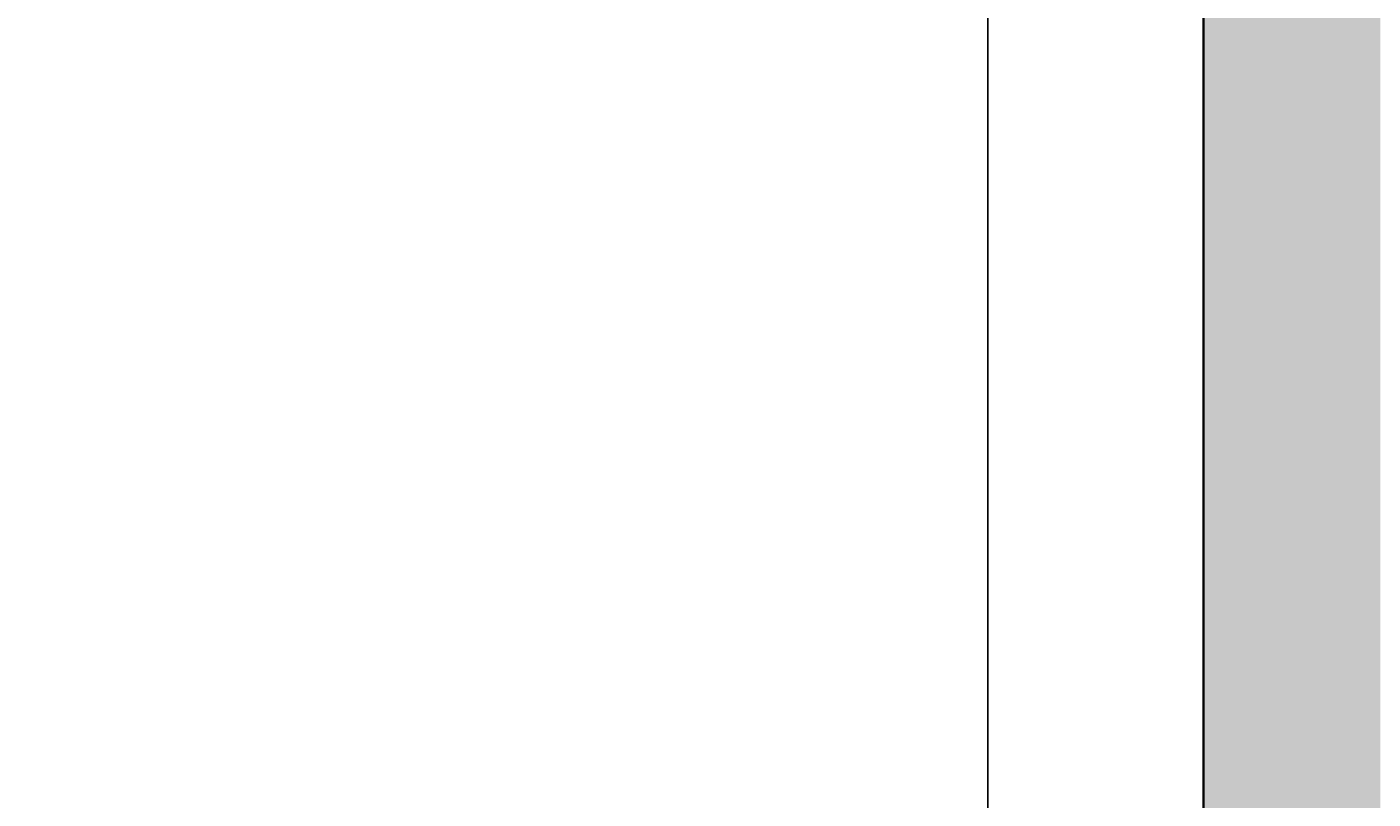
# Model space of a CAD drawing. Units: inches. Extents: x -5 to 482, y -460 to 66.
# Tile 21 of 31: x 120 to 154, y -105 to -86. Entities that reach past the tile are written whole.
import ezdxf

# ---------------------------------------------------------------- set-up
doc = ezdxf.new("R2010")
doc.units = ezdxf.units.IN
doc.header["$MEASUREMENT"] = 0
for name, color, linetype, lineweight in [('A-ANNO-DIMS', 2, 'Continuous', 18), ('A-WALL', 7, 'Continuous', 35), ('A-WALL-PATT', 152, 'Continuous', 13)]:
    doc.layers.add(name, color=color, linetype=linetype, lineweight=lineweight)
doc.styles.get("Standard").update_dxf_attribs({"font": 'arial.ttf'})
doc.dimstyles.get("Standard").update_dxf_attribs({"dimtxt": 0.18, "dimasz": 0.18, "dimexe": 0.18, "dimexo": 0.0625, "dimgap": 0.09, "dimtad": 0, "dimtih": 1, "dimtoh": 1, "dimdec": 0, "dimzin": 0, "dimdsep": 46, "dimlunit": 3, "dimtxsty": 'Standard', "dimcen": 0.09, "dimadec": 0, "dimazin": 0, "dimtfac": 1, "dimtdec": 0, "dimtofl": 0, "dimtmove": 0, "dimatfit": 3, "dimfxl": 1, "dimtolj": 1, "dimtzin": 0, "dimarcsym": 0})

# ---------------------------------------------------------------- blocks, each defined once
blk = doc.blocks.new('*D73')
at = {"layer": 'A-ANNO-DIMS', "color": 0, "lineweight": -2, "transparency": 16777216}
for p, q in [((144.377, -295.799), (144.377, 50.931)), ((144.557, 50.751), (160.976, 50.751)), ((178.197, 50.751), (161.777, 50.751)), ((178.377, -295.799), (178.377, 50.931))]:
    blk.add_line(p, q, dxfattribs=at)
at = {"layer": 'A-ANNO-DIMS', "color": 0, "transparency": 16777216}
for points in [[(144.557, 50.781), (144.557, 50.721), (144.377, 50.751)], [(178.197, 50.781), (178.197, 50.721), (178.377, 50.751)]]:
    blk.add_solid(points, dxfattribs=at)
at = {"layer": 'Defpoints', "color": 0, "transparency": 16777216}
for p in [(178.377, 50.751), (144.377, -295.861), (178.377, -295.861)]:
    blk.add_point(p, dxfattribs=at)
at = {"layer": 'A-ANNO-DIMS', "color": 0, "transparency": 16777216, "insert": (161.377, 50.751), "char_height": 0.18, "attachment_point": 5}
blk.add_mtext('\\A1;2\'-10"', dxfattribs=at)

msp = doc.modelspace()

# ---------------------------------------------------------------- hatches: boundary and pattern name
at = {"layer": 'A-WALL-PATT'}
h = msp.add_hatch(color=256, dxfattribs=at)
h.dxf.hatch_style = 1
h.paths.add_polyline_path([(149.377, -412.849), (144.377, -412.849), (144.377, -283.849), (144.377, -279.349), (133.877, -279.349), (133.877, -283.849), (139.877, -283.849), (139.877, -412.849), (133.51, -412.849), (133.51, -413.916), (102.652, -413.916), (102.652, -421.02), (133.51, -421.02), (133.51, -421.849), (149.377, -421.849)])
h.paths.add_polyline_path([(226.054, -412.849), (218.877, -412.849), (218.877, -350.849), (262.877, -350.849), (262.877, -386.849), (267.377, -386.849), (267.377, -283.849), (270.377, -283.849), (270.377, -279.349), (244.877, -279.349), (244.877, -283.849), (262.877, -283.849), (262.877, -346.349), (218.877, -346.349), (218.877, -283.849), (220.877, -283.849), (220.877, -279.349), (214.377, -279.349), (214.377, -283.849), (214.377, -412.849), (209.377, -412.849), (209.377, -421.849), (226.054, -421.849)])
h.paths.add_polyline_path([(315.815, -412.849), (250.054, -412.849), (250.054, -421.849), (315.815, -421.849)])
h.paths.add_polyline_path([(430.377, -378.349), (421.377, -378.349), (421.377, -412.849), (375.815, -412.849), (375.815, -421.849), (430.377, -421.849)])
h.paths.add_polyline_path([(78.691, -413.916), (47.68, -413.916), (47.68, -412.849), (41.877, -412.849), (41.877, -283.849), (109.877, -283.849), (109.877, -279.349), (41.877, -279.349), (41.877, -241.849), (32.877, -241.849), (32.877, -421.849), (47.68, -421.849), (47.68, -421.02), (78.691, -421.02)])
h.paths.add_polyline_path([(41.877, -144.349), (154.377, -144.349), (154.377, -137.849), (149.877, -137.849), (149.877, -139.849), (41.877, -139.849), (41.877, -97.849), (32.877, -97.849), (32.877, -181.849), (41.877, -181.849)])
h.paths.add_polyline_path([(430.377, -241.849), (421.377, -241.849), (421.377, -279.349), (309.377, -279.349), (309.377, -170.349), (304.877, -170.349), (304.877, -279.349), (294.377, -279.349), (294.377, -283.849), (421.377, -283.849), (421.377, -318.349), (430.377, -318.349)])
h.paths.add_polyline_path([(430.377, -119.849), (421.377, -119.849), (421.377, -139.849), (419.377, -139.849), (419.377, -144.349), (421.377, -144.349), (421.377, -181.849), (430.377, -181.849)])
h.paths.add_polyline_path([(395.377, -139.849), (377.377, -139.849), (377.377, -75.849), (421.377, -75.849), (421.377, -95.849), (430.377, -95.849), (430.377, -45.599), (421.377, -45.599), (421.377, -71.349), (377.377, -71.349), (377.377, -22.849), (372.877, -22.849), (372.877, -139.849), (242.877, -139.849), (242.877, -137.849), (238.377, -137.849), (238.377, -144.349), (304.877, -144.349), (304.877, -146.349), (309.377, -146.349), (309.377, -144.349), (395.377, -144.349)])
h.paths.add_polyline_path([(65.877, 13.151), (32.877, 13.151), (32.877, -37.849), (41.877, -37.849), (41.877, 4.151), (65.877, 4.151)])
h.paths.add_polyline_path([(166.377, 13.151), (125.877, 13.151), (125.877, 4.151), (149.877, 4.151), (149.877, -113.849), (154.377, -113.849), (154.377, 4.151), (166.377, 4.151)])
h.paths.add_polyline_path([(277.877, 13.151), (226.377, 13.151), (226.377, 4.151), (238.377, 4.151), (238.377, -113.849), (242.877, -113.849), (242.877, 4.151), (277.877, 4.151)])
h.paths.add_polyline_path([(430.377, 13.151), (337.877, 13.151), (337.877, 4.151), (372.877, 4.151), (372.877, 1.151), (377.377, 1.151), (377.377, 4.151), (421.377, 4.151), (421.377, -21.599), (430.377, -21.599)])

# ---------------------------------------------------------------- linework, layer by layer
at = {"layer": 'A-WALL'}
msp.add_line((149.877, 4.151), (149.877, -113.849), dxfattribs=at)

# ---------------------------------------------------------------- dimensions: what is measured, and where the dimension line sits
at = {"layer": 'A-ANNO-DIMS'}
dim = msp.add_linear_dim(base=(178.377, 50.751), p1=(144.377, -295.861), p2=(178.377, -295.861), dimstyle='Standard', override={"dimdec": 1, "dimlfac": 1, "dimrnd": 0, "dimzin": 1, "dimdsep": 46, "dimlunit": 4, "dimfrac": 2}, dxfattribs=at)
dim.commit()
dim.dimension.update_dxf_attribs({"geometry": '*D73', "text_midpoint": (161.377, 50.751)})

doc.saveas('drawing.dxf')
